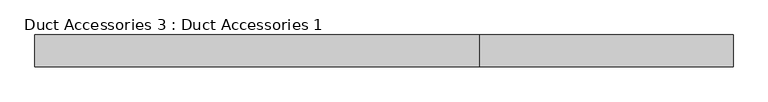
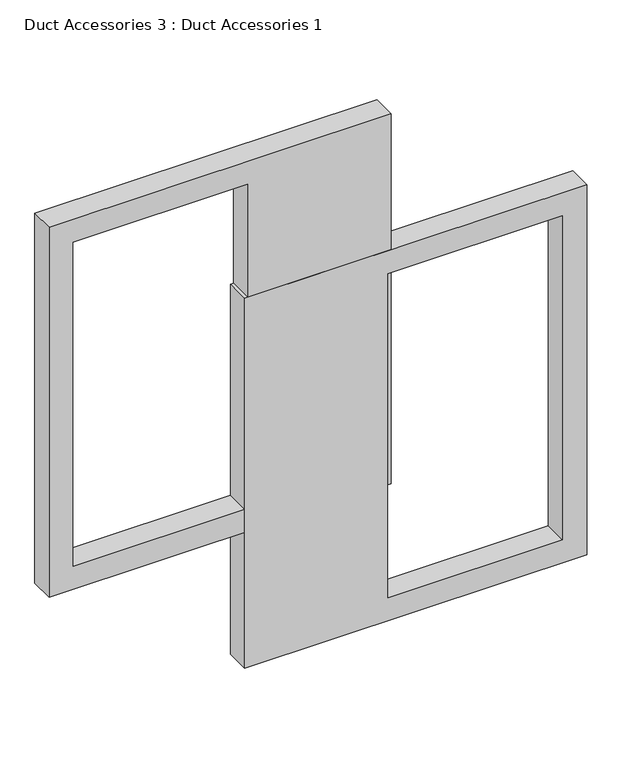
"""IFC4 building model written with IfcOpenShell, lengths in millimetres: damper geometry, Duct Accessories 3 : Duct Accessories 1."""

from ifc_helpers import new_model, si_unit, frame, origin, place, context, project, spatial, polyline, outline, extrude, source, transform, mapped, element, save


def duct_accessories_3_duct_accessories_1_969fcb05(model_context):
    return source(origin(), model_context, "Body", "SweptSolid", [
        extrude(outline(polyline([(31974.3403114, -12928.36893), (30755.1403114, -12928.36893), (30755.1403114, -11861.56893), (31974.3403114, -11861.56893), (31974.3403114, -12928.36893)]), holes=[polyline([(31898.1403114, -12480.9324751), (31898.1403114, -11937.76893), (30831.3403114, -11937.76893), (30831.3403114, -12480.9324751), (31898.1403114, -12480.9324751)])]), frame((0.0, -447.4934478, 0.0), z_axis=(0.0, 1.0, 0.0), x_axis=(0.0, 0.0, 1.0)), (0.0, 0.0, 1.0), 76.2),
        extrude(outline(polyline([(32421.7767663, -12471.5606701), (32421.7767663, -13538.3606701), (31202.5767663, -13538.3606701), (31202.5767663, -12471.5606701), (32421.7767663, -12471.5606701)]), holes=[polyline([(32345.5767663, -12918.997125), (31278.7767663, -12918.997125), (31278.7767663, -13462.1606701), (32345.5767663, -13462.1606701), (32345.5767663, -12918.997125)])]), frame((0.0, -447.4934478, 0.0), z_axis=(0.0, 1.0, 0.0), x_axis=(0.0, 0.0, 1.0)), (0.0, 0.0, 1.0), 76.2),
    ])


if __name__ == "__main__":
    model = new_model("IFC4")
    model_context = context("Model", 3, world=origin())
    ifc_project = project(units=[si_unit("LENGTHUNIT", "METRE", prefix="MILLI")], contexts=[model_context])
    site = spatial("IfcSite", under=ifc_project)
    building = spatial("IfcBuilding", under=site)
    placement = place(None, origin())
    duct_accessories_3_duct_accessories_1_shape = duct_accessories_3_duct_accessories_1_969fcb05(model_context)
    element("IfcDamper", 1, ObjectType="Duct Accessories 3 : Duct Accessories 1", at=placement, inside=building, context=model_context, shape_type="MappedRepresentation", body=[
        mapped(duct_accessories_3_duct_accessories_1_shape, transform((0.0, 0.0, 0.0), x_axis=(1.0, 0.0, 0.0), y_axis=(0.0, 1.0, 0.0), z_axis=(0.0, 0.0, 1.0))),
    ])
    save(model, "model.ifc")

# Revit data of these elements
# Element 1 (IfcDamper, "Duct Accessories 3 : Duct Accessories 1")
#   Materials on its faces: "border"
# Materials
#   "border": class "Generic", colour RGB 144 144 144, transparency 0, Cost = 0
